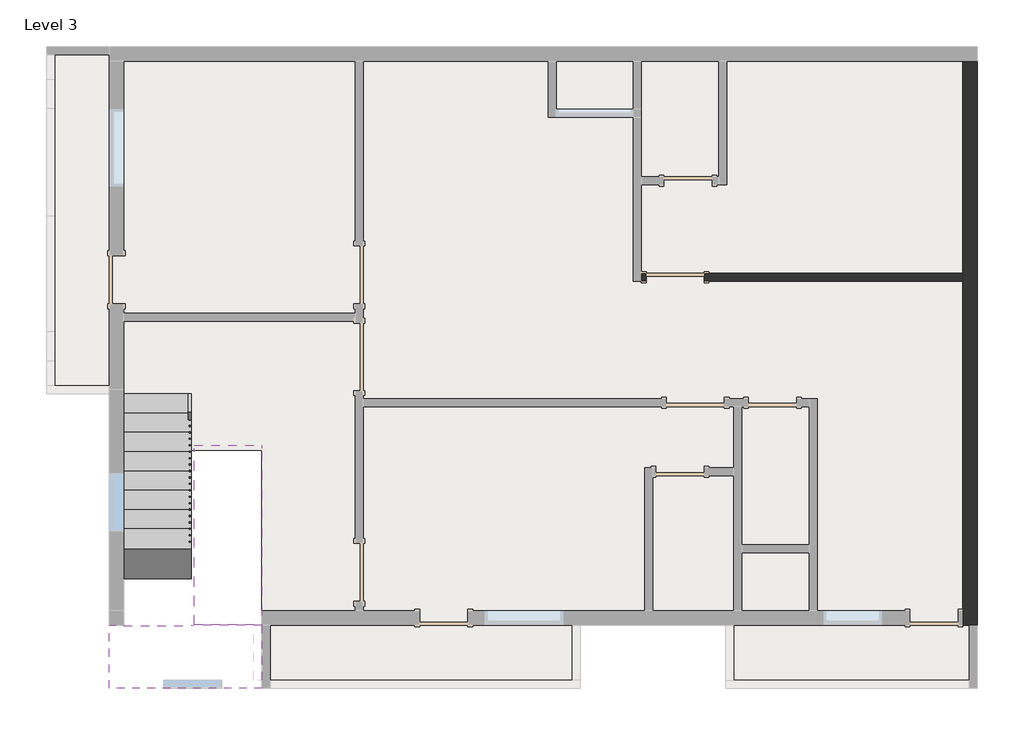
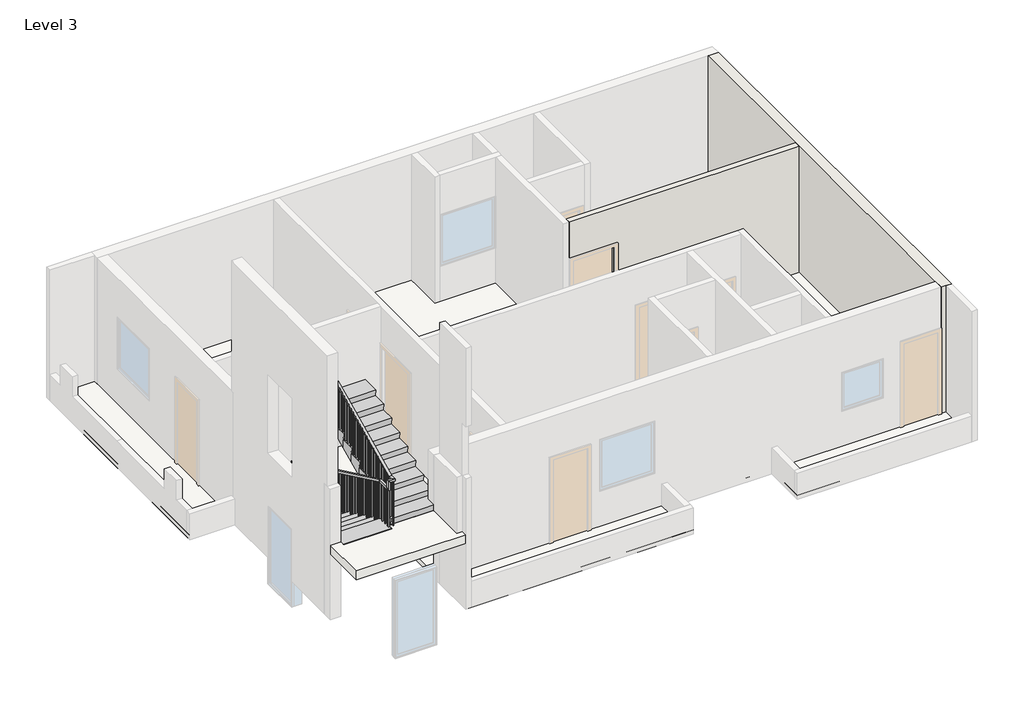
# One storey, part 2 of 2: 2 stair flights, 2 walls, 1 railing, 1 roof, 1 slab.
"""IFC4 building model written with IfcOpenShell, lengths in millimetres."""

from ifc_helpers import new_model, si_unit, frame, origin, place, context, project, spatial, polyline, outline, extrude, faceted_brep, element, save

model = new_model("IFC4")

# Units and contexts
model_context = context("Model", 3, world=origin())
ifc_project = project(units=[si_unit("LENGTHUNIT", "METRE", prefix="MILLI")], contexts=[model_context])

# Site, building, storey
site = spatial("IfcSite", under=ifc_project)
building = spatial("IfcBuilding", under=site)
storey = spatial("IfcBuildingStorey", under=building, Name="Level 3", Elevation=6096.0)

# Railing
placement = place(None, origin())
element("IfcRailing", 1, ObjectType="Handrail - Rectangular", at=placement, inside=storey, context=model_context, shape_type="SolidModel", body=[
    faceted_brep([(-9046.3394758, 7288.0495492, 7155.5428571), (-9046.3394758, 7288.0495492, 7099.2772447), (-9097.1394758, 7288.0495492, 7099.2772447), (-9097.1394758, 7288.0495492, 7155.5428571), (-9046.3394758, 3935.2495492, 8752.1142857), (-9046.3394758, 3923.7717632, 8701.3142857), (-9097.1394758, 3923.7717632, 8701.3142857), (-9097.1394758, 3935.2495492, 8752.1142857), (-9046.3394758, 3630.4495492, 8752.1142857), (-9097.1394758, 3630.4495492, 8752.1142857), (-9097.1394758, 3579.6495492, 8701.3142857), (-9046.3394758, 3579.6495492, 8701.3142857)], [[[0, 1, 2, 3]], [[1, 0, 4, 5]], [[2, 1, 5, 6]], [[3, 2, 6, 7]], [[0, 3, 7, 4]], [[8, 9, 10, 11]], [[5, 4, 8, 11]], [[6, 5, 11, 10]], [[7, 6, 10, 9]], [[4, 7, 9, 8]]]),
    faceted_brep([(-9046.3394758, 3630.4495492, 8752.1142857), (-9046.3394758, 3579.6495492, 8701.3142857), (-9097.1394758, 3579.6495492, 8701.3142857), (-9097.1394758, 3630.4495492, 8752.1142857), (-9046.3394758, 3630.4495492, 8882.7428571), (-9097.1394758, 3630.4495492, 8933.5428571), (-9097.1394758, 3579.6495492, 8933.5428571), (-9046.3394758, 3579.6495492, 8882.7428571)], [[[0, 1, 2, 3]], [[4, 5, 6, 7]], [[1, 0, 4, 7]], [[2, 1, 7, 6]], [[3, 2, 6, 5]], [[0, 3, 5, 4]]]),
    faceted_brep([(-9097.1394758, 3630.4495492, 8933.5428571), (-9046.3394758, 3630.4495492, 8882.7428571), (-9046.3394758, 3579.6495492, 8882.7428571), (-9097.1394758, 3579.6495492, 8933.5428571), (-8995.5394758, 3630.4495492, 8933.5428571), (-8995.5394758, 3630.4495492, 8882.7428571), (-8944.7394758, 3579.6495492, 8882.7428571), (-8944.7394758, 3579.6495492, 8933.5428571), (-8995.5394758, 3706.6495492, 8933.5428571), (-8995.5394758, 3718.1273353, 8882.7428571), (-8944.7394758, 3718.1273353, 8882.7428571), (-8944.7394758, 3706.6495492, 8933.5428571), (-8995.5394758, 6068.8495492, 10058.4), (-8995.5394758, 6080.3273353, 10007.6), (-8944.7394758, 6080.3273353, 10007.6), (-8944.7394758, 6068.8495492, 10058.4), (-8995.5394758, 6373.6495492, 10058.4), (-8944.7394758, 6373.6495492, 10058.4), (-8944.7394758, 6373.6495492, 10007.6), (-8995.5394758, 6373.6495492, 10007.6)], [[[0, 1, 2, 3]], [[1, 0, 4, 5]], [[2, 1, 5, 6]], [[3, 2, 6, 7]], [[0, 3, 7, 4]], [[5, 4, 8, 9]], [[6, 5, 9, 10]], [[7, 6, 10, 11]], [[4, 7, 11, 8]], [[9, 8, 12, 13]], [[10, 9, 13, 14]], [[11, 10, 14, 15]], [[8, 11, 15, 12]], [[16, 17, 18, 19]], [[13, 12, 16, 19]], [[14, 13, 19, 18]], [[15, 14, 18, 17]], [[12, 15, 17, 16]]]),
    extrude(outline(polyline([(-8979.6644758, 6338.7245492), (-8979.6644758, 6357.7745492), (-8960.6144758, 6357.7745492), (-8960.6144758, 6338.7245492), (-8979.6644758, 6338.7245492)])), frame((0.0, 0.0, 9144.0), z_axis=(0.0, 0.0, 1.0), x_axis=(1.0, 0.0, 0.0)), (0.0, 0.0, 1.0), 863.6),
    extrude(outline(polyline([(-8979.6644758, 6237.1245492), (-8979.6644758, 6256.1745492), (-8960.6144758, 6256.1745492), (-8960.6144758, 6237.1245492), (-8979.6644758, 6237.1245492)])), frame((0.0, 0.0, 9144.0), z_axis=(0.0, 0.0, 1.0), x_axis=(1.0, 0.0, 0.0)), (0.0, 0.0, 1.0), 863.6),
    extrude(outline(polyline([(-8979.6644758, 6135.5245492), (-8979.6644758, 6154.5745492), (-8960.6144758, 6154.5745492), (-8960.6144758, 6135.5245492), (-8979.6644758, 6135.5245492)])), frame((0.0, 0.0, 9144.0), z_axis=(0.0, 0.0, 1.0), x_axis=(1.0, 0.0, 0.0)), (0.0, 0.0, 1.0), 863.6),
    extrude(outline(polyline([(6052.9745492, 9994.5748638), (6052.9745492, 8998.8571429), (6033.9245492, 8998.8571429), (6033.9245492, 9985.5034352), (6052.9745492, 9994.5748638)])), frame((-8979.6644758, 0.0, 0.0), z_axis=(1.0, 0.0, 0.0), x_axis=(0.0, 1.0, 0.0)), (0.0, 0.0, 1.0), 19.05),
    extrude(outline(polyline([(5951.3745492, 9946.1939114), (5951.3745492, 8998.8571429), (5932.3245492, 8998.8571429), (5932.3245492, 9937.1224828), (5951.3745492, 9946.1939114)])), frame((-8979.6644758, 0.0, 0.0), z_axis=(1.0, 0.0, 0.0), x_axis=(0.0, 1.0, 0.0)), (0.0, 0.0, 1.0), 19.05),
    extrude(outline(polyline([(5849.7745492, 9897.812959), (5849.7745492, 8998.8571429), (5830.7245492, 8998.8571429), (5830.7245492, 9888.7415305), (5849.7745492, 9897.812959)])), frame((-8979.6644758, 0.0, 0.0), z_axis=(1.0, 0.0, 0.0), x_axis=(0.0, 1.0, 0.0)), (0.0, 0.0, 1.0), 19.05),
    extrude(outline(polyline([(5748.1745492, 9849.4320067), (5748.1745492, 8853.7142857), (5729.1245492, 8853.7142857), (5729.1245492, 9840.3605781), (5748.1745492, 9849.4320067)])), frame((-8979.6644758, 0.0, 0.0), z_axis=(1.0, 0.0, 0.0), x_axis=(0.0, 1.0, 0.0)), (0.0, 0.0, 1.0), 19.05),
    extrude(outline(polyline([(5646.5745492, 9801.0510543), (5646.5745492, 8853.7142857), (5627.5245492, 8853.7142857), (5627.5245492, 9791.9796257), (5646.5745492, 9801.0510543)])), frame((-8979.6644758, 0.0, 0.0), z_axis=(1.0, 0.0, 0.0), x_axis=(0.0, 1.0, 0.0)), (0.0, 0.0, 1.0), 19.05),
    extrude(outline(polyline([(5544.9745492, 9752.6701019), (5544.9745492, 8853.7142857), (5525.9245492, 8853.7142857), (5525.9245492, 9743.5986733), (5544.9745492, 9752.6701019)])), frame((-8979.6644758, 0.0, 0.0), z_axis=(1.0, 0.0, 0.0), x_axis=(0.0, 1.0, 0.0)), (0.0, 0.0, 1.0), 19.05),
    extrude(outline(polyline([(5443.3745492, 9704.2891495), (5443.3745492, 8708.5714286), (5424.3245492, 8708.5714286), (5424.3245492, 9695.2177209), (5443.3745492, 9704.2891495)])), frame((-8979.6644758, 0.0, 0.0), z_axis=(1.0, 0.0, 0.0), x_axis=(0.0, 1.0, 0.0)), (0.0, 0.0, 1.0), 19.05),
    extrude(outline(polyline([(5341.7745492, 9655.9081971), (5341.7745492, 8708.5714286), (5322.7245492, 8708.5714286), (5322.7245492, 9646.8367686), (5341.7745492, 9655.9081971)])), frame((-8979.6644758, 0.0, 0.0), z_axis=(1.0, 0.0, 0.0), x_axis=(0.0, 1.0, 0.0)), (0.0, 0.0, 1.0), 19.05),
    extrude(outline(polyline([(5240.1745492, 9607.5272447), (5240.1745492, 8708.5714286), (5221.1245492, 8708.5714286), (5221.1245492, 9598.4558162), (5240.1745492, 9607.5272447)])), frame((-8979.6644758, 0.0, 0.0), z_axis=(1.0, 0.0, 0.0), x_axis=(0.0, 1.0, 0.0)), (0.0, 0.0, 1.0), 19.05),
    extrude(outline(polyline([(5138.5745492, 9559.1462924), (5138.5745492, 8563.4285714), (5119.5245492, 8563.4285714), (5119.5245492, 9550.0748638), (5138.5745492, 9559.1462924)])), frame((-8979.6644758, 0.0, 0.0), z_axis=(1.0, 0.0, 0.0), x_axis=(0.0, 1.0, 0.0)), (0.0, 0.0, 1.0), 19.05),
    extrude(outline(polyline([(5036.9745492, 9510.76534), (5036.9745492, 8563.4285714), (5017.9245492, 8563.4285714), (5017.9245492, 9501.6939114), (5036.9745492, 9510.76534)])), frame((-8979.6644758, 0.0, 0.0), z_axis=(1.0, 0.0, 0.0), x_axis=(0.0, 1.0, 0.0)), (0.0, 0.0, 1.0), 19.05),
    extrude(outline(polyline([(4935.3745492, 9462.3843876), (4935.3745492, 8563.4285714), (4916.3245492, 8563.4285714), (4916.3245492, 9453.312959), (4935.3745492, 9462.3843876)])), frame((-8979.6644758, 0.0, 0.0), z_axis=(1.0, 0.0, 0.0), x_axis=(0.0, 1.0, 0.0)), (0.0, 0.0, 1.0), 19.05),
    extrude(outline(polyline([(4833.7745492, 9414.0034352), (4833.7745492, 8418.2857143), (4814.7245492, 8418.2857143), (4814.7245492, 9404.9320067), (4833.7745492, 9414.0034352)])), frame((-8979.6644758, 0.0, 0.0), z_axis=(1.0, 0.0, 0.0), x_axis=(0.0, 1.0, 0.0)), (0.0, 0.0, 1.0), 19.05),
    extrude(outline(polyline([(4732.1745492, 9365.6224828), (4732.1745492, 8418.2857143), (4713.1245492, 8418.2857143), (4713.1245492, 9356.5510543), (4732.1745492, 9365.6224828)])), frame((-8979.6644758, 0.0, 0.0), z_axis=(1.0, 0.0, 0.0), x_axis=(0.0, 1.0, 0.0)), (0.0, 0.0, 1.0), 19.05),
    extrude(outline(polyline([(4630.5745492, 9317.2415305), (4630.5745492, 8418.2857143), (4611.5245492, 8418.2857143), (4611.5245492, 9308.1701019), (4630.5745492, 9317.2415305)])), frame((-8979.6644758, 0.0, 0.0), z_axis=(1.0, 0.0, 0.0), x_axis=(0.0, 1.0, 0.0)), (0.0, 0.0, 1.0), 19.05),
    extrude(outline(polyline([(4528.9745492, 9268.8605781), (4528.9745492, 8273.1428571), (4509.9245492, 8273.1428571), (4509.9245492, 9259.7891495), (4528.9745492, 9268.8605781)])), frame((-8979.6644758, 0.0, 0.0), z_axis=(1.0, 0.0, 0.0), x_axis=(0.0, 1.0, 0.0)), (0.0, 0.0, 1.0), 19.05),
    extrude(outline(polyline([(4427.3745492, 9220.4796257), (4427.3745492, 8273.1428571), (4408.3245492, 8273.1428571), (4408.3245492, 9211.4081971), (4427.3745492, 9220.4796257)])), frame((-8979.6644758, 0.0, 0.0), z_axis=(1.0, 0.0, 0.0), x_axis=(0.0, 1.0, 0.0)), (0.0, 0.0, 1.0), 19.05),
    extrude(outline(polyline([(4325.7745492, 9172.0986733), (4325.7745492, 8273.1428571), (4306.7245492, 8273.1428571), (4306.7245492, 9163.0272447), (4325.7745492, 9172.0986733)])), frame((-8979.6644758, 0.0, 0.0), z_axis=(1.0, 0.0, 0.0), x_axis=(0.0, 1.0, 0.0)), (0.0, 0.0, 1.0), 19.05),
    extrude(outline(polyline([(4224.1745492, 9123.7177209), (4224.1745492, 8128.0), (4205.1245492, 8128.0), (4205.1245492, 9114.6462924), (4224.1745492, 9123.7177209)])), frame((-8979.6644758, 0.0, 0.0), z_axis=(1.0, 0.0, 0.0), x_axis=(0.0, 1.0, 0.0)), (0.0, 0.0, 1.0), 19.05),
    extrude(outline(polyline([(4122.5745492, 9075.3367686), (4122.5745492, 8128.0), (4103.5245492, 8128.0), (4103.5245492, 9066.26534), (4122.5745492, 9075.3367686)])), frame((-8979.6644758, 0.0, 0.0), z_axis=(1.0, 0.0, 0.0), x_axis=(0.0, 1.0, 0.0)), (0.0, 0.0, 1.0), 19.05),
    extrude(outline(polyline([(4020.9745492, 9026.9558162), (4020.9745492, 8128.0), (4001.9245492, 8128.0), (4001.9245492, 9017.8843876), (4020.9745492, 9026.9558162)])), frame((-8979.6644758, 0.0, 0.0), z_axis=(1.0, 0.0, 0.0), x_axis=(0.0, 1.0, 0.0)), (0.0, 0.0, 1.0), 19.05),
    extrude(outline(polyline([(3919.3745492, 8978.5748638), (3919.3745492, 7982.8571429), (3900.3245492, 7982.8571429), (3900.3245492, 8969.5034352), (3919.3745492, 8978.5748638)])), frame((-8979.6644758, 0.0, 0.0), z_axis=(1.0, 0.0, 0.0), x_axis=(0.0, 1.0, 0.0)), (0.0, 0.0, 1.0), 19.05),
    extrude(outline(polyline([(3817.7745492, 8930.1939114), (3817.7745492, 7982.8571429), (3798.7245492, 7982.8571429), (3798.7245492, 8921.1224828), (3817.7745492, 8930.1939114)])), frame((-8979.6644758, 0.0, 0.0), z_axis=(1.0, 0.0, 0.0), x_axis=(0.0, 1.0, 0.0)), (0.0, 0.0, 1.0), 19.05),
    extrude(outline(polyline([(3716.1745492, 8881.812959), (3716.1745492, 7982.8571429), (3697.1245492, 7982.8571429), (3697.1245492, 8872.7415305), (3716.1745492, 8881.812959)])), frame((-8979.6644758, 0.0, 0.0), z_axis=(1.0, 0.0, 0.0), x_axis=(0.0, 1.0, 0.0)), (0.0, 0.0, 1.0), 19.05),
    extrude(outline(polyline([(-9062.2144758, 3639.9745492), (-9062.2144758, 3620.9245492), (-9081.2644758, 3620.9245492), (-9081.2644758, 3639.9745492), (-9062.2144758, 3639.9745492)])), frame((0.0, 0.0, 7837.7142857), z_axis=(0.0, 0.0, 1.0), x_axis=(1.0, 0.0, 0.0)), (0.0, 0.0, 1.0), 863.6),
    extrude(outline(polyline([(-9062.2144758, 3741.5745492), (-9062.2144758, 3722.5245492), (-9081.2644758, 3722.5245492), (-9081.2644758, 3741.5745492), (-9062.2144758, 3741.5745492)])), frame((0.0, 0.0, 7837.7142857), z_axis=(0.0, 0.0, 1.0), x_axis=(1.0, 0.0, 0.0)), (0.0, 0.0, 1.0), 863.6),
    extrude(outline(polyline([(-9062.2144758, 3843.1745492), (-9062.2144758, 3824.1245492), (-9081.2644758, 3824.1245492), (-9081.2644758, 3843.1745492), (-9062.2144758, 3843.1745492)])), frame((0.0, 0.0, 7837.7142857), z_axis=(0.0, 0.0, 1.0), x_axis=(1.0, 0.0, 0.0)), (0.0, 0.0, 1.0), 863.6),
    extrude(outline(polyline([(3944.7745492, 8691.312959), (3944.7745492, 7837.7142857), (3925.7245492, 7837.7142857), (3925.7245492, 8700.3843876), (3944.7745492, 8691.312959)])), frame((-9081.2644758, 0.0, 0.0), z_axis=(1.0, 0.0, 0.0), x_axis=(0.0, 1.0, 0.0)), (0.0, 0.0, 1.0), 19.05),
    extrude(outline(polyline([(4046.3745492, 8642.9320067), (4046.3745492, 7692.5714286), (4027.3245492, 7692.5714286), (4027.3245492, 8652.0034352), (4046.3745492, 8642.9320067)])), frame((-9081.2644758, 0.0, 0.0), z_axis=(1.0, 0.0, 0.0), x_axis=(0.0, 1.0, 0.0)), (0.0, 0.0, 1.0), 19.05),
    extrude(outline(polyline([(4147.9745492, 8594.5510543), (4147.9745492, 7692.5714286), (4128.9245492, 7692.5714286), (4128.9245492, 8603.6224828), (4147.9745492, 8594.5510543)])), frame((-9081.2644758, 0.0, 0.0), z_axis=(1.0, 0.0, 0.0), x_axis=(0.0, 1.0, 0.0)), (0.0, 0.0, 1.0), 19.05),
    extrude(outline(polyline([(4249.5745492, 8546.1701019), (4249.5745492, 7692.5714286), (4230.5245492, 7692.5714286), (4230.5245492, 8555.2415305), (4249.5745492, 8546.1701019)])), frame((-9081.2644758, 0.0, 0.0), z_axis=(1.0, 0.0, 0.0), x_axis=(0.0, 1.0, 0.0)), (0.0, 0.0, 1.0), 19.05),
    extrude(outline(polyline([(4351.1745492, 8497.7891495), (4351.1745492, 7547.4285714), (4332.1245492, 7547.4285714), (4332.1245492, 8506.8605781), (4351.1745492, 8497.7891495)])), frame((-9081.2644758, 0.0, 0.0), z_axis=(1.0, 0.0, 0.0), x_axis=(0.0, 1.0, 0.0)), (0.0, 0.0, 1.0), 19.05),
    extrude(outline(polyline([(4452.7745492, 8449.4081971), (4452.7745492, 7547.4285714), (4433.7245492, 7547.4285714), (4433.7245492, 8458.4796257), (4452.7745492, 8449.4081971)])), frame((-9081.2644758, 0.0, 0.0), z_axis=(1.0, 0.0, 0.0), x_axis=(0.0, 1.0, 0.0)), (0.0, 0.0, 1.0), 19.05),
    extrude(outline(polyline([(4554.3745492, 8401.0272447), (4554.3745492, 7547.4285714), (4535.3245492, 7547.4285714), (4535.3245492, 8410.0986733), (4554.3745492, 8401.0272447)])), frame((-9081.2644758, 0.0, 0.0), z_axis=(1.0, 0.0, 0.0), x_axis=(0.0, 1.0, 0.0)), (0.0, 0.0, 1.0), 19.05),
    extrude(outline(polyline([(4655.9745492, 8352.6462924), (4655.9745492, 7402.2857143), (4636.9245492, 7402.2857143), (4636.9245492, 8361.7177209), (4655.9745492, 8352.6462924)])), frame((-9081.2644758, 0.0, 0.0), z_axis=(1.0, 0.0, 0.0), x_axis=(0.0, 1.0, 0.0)), (0.0, 0.0, 1.0), 19.05),
    extrude(outline(polyline([(4757.5745492, 8304.26534), (4757.5745492, 7402.2857143), (4738.5245492, 7402.2857143), (4738.5245492, 8313.3367686), (4757.5745492, 8304.26534)])), frame((-9081.2644758, 0.0, 0.0), z_axis=(1.0, 0.0, 0.0), x_axis=(0.0, 1.0, 0.0)), (0.0, 0.0, 1.0), 19.05),
    extrude(outline(polyline([(4859.1745492, 8255.8843876), (4859.1745492, 7402.2857143), (4840.1245492, 7402.2857143), (4840.1245492, 8264.9558162), (4859.1745492, 8255.8843876)])), frame((-9081.2644758, 0.0, 0.0), z_axis=(1.0, 0.0, 0.0), x_axis=(0.0, 1.0, 0.0)), (0.0, 0.0, 1.0), 19.05),
    extrude(outline(polyline([(4960.7745492, 8207.5034352), (4960.7745492, 7257.1428571), (4941.7245492, 7257.1428571), (4941.7245492, 8216.5748638), (4960.7745492, 8207.5034352)])), frame((-9081.2644758, 0.0, 0.0), z_axis=(1.0, 0.0, 0.0), x_axis=(0.0, 1.0, 0.0)), (0.0, 0.0, 1.0), 19.05),
    extrude(outline(polyline([(5062.3745492, 8159.1224828), (5062.3745492, 7257.1428571), (5043.3245492, 7257.1428571), (5043.3245492, 8168.1939114), (5062.3745492, 8159.1224828)])), frame((-9081.2644758, 0.0, 0.0), z_axis=(1.0, 0.0, 0.0), x_axis=(0.0, 1.0, 0.0)), (0.0, 0.0, 1.0), 19.05),
    extrude(outline(polyline([(5163.9745492, 8110.7415305), (5163.9745492, 7257.1428571), (5144.9245492, 7257.1428571), (5144.9245492, 8119.812959), (5163.9745492, 8110.7415305)])), frame((-9081.2644758, 0.0, 0.0), z_axis=(1.0, 0.0, 0.0), x_axis=(0.0, 1.0, 0.0)), (0.0, 0.0, 1.0), 19.05),
    extrude(outline(polyline([(5265.5745492, 8062.3605781), (5265.5745492, 7112.0), (5246.5245492, 7112.0), (5246.5245492, 8071.4320067), (5265.5745492, 8062.3605781)])), frame((-9081.2644758, 0.0, 0.0), z_axis=(1.0, 0.0, 0.0), x_axis=(0.0, 1.0, 0.0)), (0.0, 0.0, 1.0), 19.05),
    extrude(outline(polyline([(5367.1745492, 8013.9796257), (5367.1745492, 7112.0), (5348.1245492, 7112.0), (5348.1245492, 8023.0510543), (5367.1745492, 8013.9796257)])), frame((-9081.2644758, 0.0, 0.0), z_axis=(1.0, 0.0, 0.0), x_axis=(0.0, 1.0, 0.0)), (0.0, 0.0, 1.0), 19.05),
    extrude(outline(polyline([(5468.7745492, 7965.5986733), (5468.7745492, 7112.0), (5449.7245492, 7112.0), (5449.7245492, 7974.6701019), (5468.7745492, 7965.5986733)])), frame((-9081.2644758, 0.0, 0.0), z_axis=(1.0, 0.0, 0.0), x_axis=(0.0, 1.0, 0.0)), (0.0, 0.0, 1.0), 19.05),
    extrude(outline(polyline([(5570.3745492, 7917.2177209), (5570.3745492, 6966.8571429), (5551.3245492, 6966.8571429), (5551.3245492, 7926.2891495), (5570.3745492, 7917.2177209)])), frame((-9081.2644758, 0.0, 0.0), z_axis=(1.0, 0.0, 0.0), x_axis=(0.0, 1.0, 0.0)), (0.0, 0.0, 1.0), 19.05),
    extrude(outline(polyline([(5671.9745492, 7868.8367686), (5671.9745492, 6966.8571429), (5652.9245492, 6966.8571429), (5652.9245492, 7877.9081971), (5671.9745492, 7868.8367686)])), frame((-9081.2644758, 0.0, 0.0), z_axis=(1.0, 0.0, 0.0), x_axis=(0.0, 1.0, 0.0)), (0.0, 0.0, 1.0), 19.05),
    extrude(outline(polyline([(5773.5745492, 7820.4558162), (5773.5745492, 6966.8571429), (5754.5245492, 6966.8571429), (5754.5245492, 7829.5272447), (5773.5745492, 7820.4558162)])), frame((-9081.2644758, 0.0, 0.0), z_axis=(1.0, 0.0, 0.0), x_axis=(0.0, 1.0, 0.0)), (0.0, 0.0, 1.0), 19.05),
    extrude(outline(polyline([(5875.1745492, 7772.0748638), (5875.1745492, 6821.7142857), (5856.1245492, 6821.7142857), (5856.1245492, 7781.1462924), (5875.1745492, 7772.0748638)])), frame((-9081.2644758, 0.0, 0.0), z_axis=(1.0, 0.0, 0.0), x_axis=(0.0, 1.0, 0.0)), (0.0, 0.0, 1.0), 19.05),
    extrude(outline(polyline([(5976.7745492, 7723.6939114), (5976.7745492, 6821.7142857), (5957.7245492, 6821.7142857), (5957.7245492, 7732.76534), (5976.7745492, 7723.6939114)])), frame((-9081.2644758, 0.0, 0.0), z_axis=(1.0, 0.0, 0.0), x_axis=(0.0, 1.0, 0.0)), (0.0, 0.0, 1.0), 19.05),
    extrude(outline(polyline([(6078.3745492, 7675.312959), (6078.3745492, 6821.7142857), (6059.3245492, 6821.7142857), (6059.3245492, 7684.3843876), (6078.3745492, 7675.312959)])), frame((-9081.2644758, 0.0, 0.0), z_axis=(1.0, 0.0, 0.0), x_axis=(0.0, 1.0, 0.0)), (0.0, 0.0, 1.0), 19.05),
    extrude(outline(polyline([(6179.9745492, 7626.9320067), (6179.9745492, 6676.5714286), (6160.9245492, 6676.5714286), (6160.9245492, 7636.0034352), (6179.9745492, 7626.9320067)])), frame((-9081.2644758, 0.0, 0.0), z_axis=(1.0, 0.0, 0.0), x_axis=(0.0, 1.0, 0.0)), (0.0, 0.0, 1.0), 19.05),
    extrude(outline(polyline([(6281.5745492, 7578.5510543), (6281.5745492, 6676.5714286), (6262.5245492, 6676.5714286), (6262.5245492, 7587.6224828), (6281.5745492, 7578.5510543)])), frame((-9081.2644758, 0.0, 0.0), z_axis=(1.0, 0.0, 0.0), x_axis=(0.0, 1.0, 0.0)), (0.0, 0.0, 1.0), 19.05),
    extrude(outline(polyline([(6383.1745492, 7530.1701019), (6383.1745492, 6676.5714286), (6364.1245492, 6676.5714286), (6364.1245492, 7539.2415305), (6383.1745492, 7530.1701019)])), frame((-9081.2644758, 0.0, 0.0), z_axis=(1.0, 0.0, 0.0), x_axis=(0.0, 1.0, 0.0)), (0.0, 0.0, 1.0), 19.05),
    extrude(outline(polyline([(6484.7745492, 7481.7891495), (6484.7745492, 6531.4285714), (6465.7245492, 6531.4285714), (6465.7245492, 7490.8605781), (6484.7745492, 7481.7891495)])), frame((-9081.2644758, 0.0, 0.0), z_axis=(1.0, 0.0, 0.0), x_axis=(0.0, 1.0, 0.0)), (0.0, 0.0, 1.0), 19.05),
    extrude(outline(polyline([(6586.3745492, 7433.4081971), (6586.3745492, 6531.4285714), (6567.3245492, 6531.4285714), (6567.3245492, 7442.4796257), (6586.3745492, 7433.4081971)])), frame((-9081.2644758, 0.0, 0.0), z_axis=(1.0, 0.0, 0.0), x_axis=(0.0, 1.0, 0.0)), (0.0, 0.0, 1.0), 19.05),
    extrude(outline(polyline([(6687.9745492, 7385.0272447), (6687.9745492, 6531.4285714), (6668.9245492, 6531.4285714), (6668.9245492, 7394.0986733), (6687.9745492, 7385.0272447)])), frame((-9081.2644758, 0.0, 0.0), z_axis=(1.0, 0.0, 0.0), x_axis=(0.0, 1.0, 0.0)), (0.0, 0.0, 1.0), 19.05),
    extrude(outline(polyline([(6789.5745492, 7336.6462924), (6789.5745492, 6386.2857143), (6770.5245492, 6386.2857143), (6770.5245492, 7345.7177209), (6789.5745492, 7336.6462924)])), frame((-9081.2644758, 0.0, 0.0), z_axis=(1.0, 0.0, 0.0), x_axis=(0.0, 1.0, 0.0)), (0.0, 0.0, 1.0), 19.05),
    extrude(outline(polyline([(6891.1745492, 7288.26534), (6891.1745492, 6386.2857143), (6872.1245492, 6386.2857143), (6872.1245492, 7297.3367686), (6891.1745492, 7288.26534)])), frame((-9081.2644758, 0.0, 0.0), z_axis=(1.0, 0.0, 0.0), x_axis=(0.0, 1.0, 0.0)), (0.0, 0.0, 1.0), 19.05),
    extrude(outline(polyline([(6992.7745492, 7239.8843876), (6992.7745492, 6386.2857143), (6973.7245492, 6386.2857143), (6973.7245492, 7248.9558162), (6992.7745492, 7239.8843876)])), frame((-9081.2644758, 0.0, 0.0), z_axis=(1.0, 0.0, 0.0), x_axis=(0.0, 1.0, 0.0)), (0.0, 0.0, 1.0), 19.05),
    extrude(outline(polyline([(7094.3745492, 7191.5034352), (7094.3745492, 6241.1428571), (7075.3245492, 6241.1428571), (7075.3245492, 7200.5748638), (7094.3745492, 7191.5034352)])), frame((-9081.2644758, 0.0, 0.0), z_axis=(1.0, 0.0, 0.0), x_axis=(0.0, 1.0, 0.0)), (0.0, 0.0, 1.0), 19.05),
    extrude(outline(polyline([(7195.9745492, 7143.1224828), (7195.9745492, 6241.1428571), (7176.9245492, 6241.1428571), (7176.9245492, 7152.1939114), (7195.9745492, 7143.1224828)])), frame((-9081.2644758, 0.0, 0.0), z_axis=(1.0, 0.0, 0.0), x_axis=(0.0, 1.0, 0.0)), (0.0, 0.0, 1.0), 19.05),
    extrude(outline(polyline([(-8979.6644758, 3614.5745492), (-8960.6144758, 3614.5745492), (-8960.6144758, 3595.5245492), (-8979.6644758, 3595.5245492), (-8979.6644758, 3614.5745492)])), frame((0.0, 0.0, 7837.7142857), z_axis=(0.0, 0.0, 1.0), x_axis=(1.0, 0.0, 0.0)), (0.0, 0.0, 1.0), 1045.0285714),
    extrude(outline(polyline([(-9062.2144758, 3614.5745492), (-9062.2144758, 3595.5245492), (-9081.2644758, 3595.5245492), (-9081.2644758, 3614.5745492), (-9062.2144758, 3614.5745492)])), frame((0.0, 0.0, 7837.7142857), z_axis=(0.0, 0.0, 1.0), x_axis=(1.0, 0.0, 0.0)), (0.0, 0.0, 1.0), 863.6),
    extrude(outline(polyline([(-8979.6644758, 6354.5995492), (-8979.6644758, 6373.6495492), (-8960.6144758, 6373.6495492), (-8960.6144758, 6354.5995492), (-8979.6644758, 6354.5995492)])), frame((0.0, 0.0, 9144.0), z_axis=(0.0, 0.0, 1.0), x_axis=(1.0, 0.0, 0.0)), (0.0, 0.0, 1.0), 863.6),
    extrude(outline(polyline([(7288.0495492, 7099.2772447), (7288.0495492, 6241.1428571), (7268.9995492, 6241.1428571), (7268.9995492, 7108.3486733), (7288.0495492, 7099.2772447)])), frame((-9081.2644758, 0.0, 0.0), z_axis=(1.0, 0.0, 0.0), x_axis=(0.0, 1.0, 0.0)), (0.0, 0.0, 1.0), 19.05),
])

# Roof
element("IfcRoof", 2, ObjectType="Generic - 4\"", at=placement, inside=storey, context=model_context, shape_type="SweptSolid", body=[
    extrude(outline(polyline([(3374.2605242, 2639.8495492), (-600.8394758, 2639.8495492), (-600.8394758, 3630.4495492), (-2899.5394758, 3630.4495492), (-2899.5394758, 2639.8495492), (-7928.7394758, 2639.8495492), (-7928.7394758, 6399.0495492), (-9046.3394758, 6399.0495492), (-9046.3394758, 7288.0495492), (-11332.3394758, 7288.0495492), (-11332.3394758, 12774.4495492), (3374.2605242, 12774.4495492), (3374.2605242, 2639.8495492)])), frame((0.0, 0.0, 6096.0), z_axis=(0.0, 0.0, 1.0), x_axis=(1.0, 0.0, 0.0)), (0.0, 0.0, 1.0), 101.6),
])

# Slab
element("IfcSlab", 3, ObjectType="8\" Thickness", at=placement, inside=storey, context=model_context, shape_type="Brep", body=[
    faceted_brep([(-10341.7394758, 3630.4495492, 7837.7142857), (-10341.7394758, 2639.8495492, 7837.7142857), (-7928.7394758, 2639.8495492, 7837.7142857), (-7928.7394758, 3630.4495492, 7837.7142857), (-7928.7394758, 3649.4995492, 7837.7142857), (-8995.5394758, 3649.4995492, 7837.7142857), (-8995.5394758, 3630.4495492, 7837.7142857), (-9044.7519758, 3630.4495492, 7837.7142857), (-9044.7519758, 3519.3245492, 7837.7142857), (-10114.7269758, 3519.3245492, 7837.7142857), (-10114.7269758, 3630.4495492, 7837.7142857), (-10341.7394758, 3630.4495492, 7634.5142857), (-10341.7394758, 2639.8495492, 7634.5142857), (-7928.7394758, 2639.8495492, 7634.5142857), (-10114.7269758, 3630.4495492, 7634.5142857), (-10114.7269758, 3620.9245492, 7634.5142857), (-9044.7519758, 3620.9245492, 7634.5142857), (-9044.7519758, 3630.4495492, 7634.5142857), (-8995.5394758, 3630.4495492, 7634.5142857), (-8995.5394758, 3649.4995492, 7634.5142857), (-7928.7394758, 3649.4995492, 7634.5142857), (-7928.7394758, 3630.4495492, 7634.5142857), (-10114.7269758, 3519.3245492, 7726.5892857), (-9044.7519758, 3519.3245492, 7726.5892857), (-9044.7519758, 3620.9245492, 7726.5892857), (-10114.7269758, 3620.9245492, 7726.5892857)], [[[0, 1, 2, 3, 4, 5, 6, 7, 8, 9, 10]], [[1, 0, 11, 12]], [[2, 1, 12, 13]], [[12, 11, 14, 15, 16, 17, 18, 19, 20, 21, 13]], [[3, 2, 13, 21]], [[5, 4, 20, 19]], [[6, 18, 17, 7]], [[22, 23, 24, 25]], [[9, 22, 25, 15, 14, 10]], [[23, 22, 9, 8]], [[23, 8, 7, 17, 16, 24]], [[25, 24, 16, 15]], [[11, 0, 10, 14]], [[4, 3, 21, 20]], [[6, 5, 19, 18]]]),
])

# Stair flights
element("IfcStairFlight", 4, ObjectType="3/4\" Nosing 6 1/2\" Depth", at=placement, inside=storey, context=model_context, shape_type="Brep", body=[
    faceted_brep([(-10113.1394758, 7288.0495492, 6241.1428571), (-9046.3394758, 7288.0495492, 6241.1428571), (-9046.3394758, 7268.9995492, 6096.0), (-10113.1394758, 7268.9995492, 6096.0), (-10113.1394758, 6964.1995492, 6241.1428571), (-9046.3394758, 6964.1995492, 6241.1428571), (-9046.3394758, 6964.1995492, 6096.0), (-10113.1394758, 6964.1995492, 6096.0), (-9046.3394758, 6983.2495492, 6386.2857143), (-10113.1394758, 6983.2495492, 6386.2857143), (-10113.1394758, 6659.3995492, 6386.2857143), (-9046.3394758, 6659.3995492, 6386.2857143), (-9046.3394758, 6659.3995492, 6203.422474), (-9046.3394758, 6884.9867446, 6096.0), (-10113.1394758, 6884.9867446, 6096.0), (-10113.1394758, 6659.3995492, 6203.422474), (-9046.3394758, 6678.4495492, 6531.4285714), (-10113.1394758, 6678.4495492, 6531.4285714), (-10113.1394758, 6354.5995492, 6531.4285714), (-9046.3394758, 6354.5995492, 6531.4285714), (-9046.3394758, 6354.5995492, 6348.5653311), (-10113.1394758, 6354.5995492, 6348.5653311), (-9046.3394758, 6373.6495492, 6676.5714286), (-10113.1394758, 6373.6495492, 6676.5714286), (-10113.1394758, 6049.7995492, 6676.5714286), (-9046.3394758, 6049.7995492, 6676.5714286), (-9046.3394758, 6049.7995492, 6493.7081883), (-10113.1394758, 6049.7995492, 6493.7081883), (-9046.3394758, 6068.8495492, 6821.7142857), (-10113.1394758, 6068.8495492, 6821.7142857), (-10113.1394758, 5744.9995492, 6821.7142857), (-9046.3394758, 5744.9995492, 6821.7142857), (-9046.3394758, 5744.9995492, 6638.8510454), (-10113.1394758, 5744.9995492, 6638.8510454), (-9046.3394758, 5764.0495492, 6966.8571429), (-10113.1394758, 5764.0495492, 6966.8571429), (-10113.1394758, 5440.1995492, 6966.8571429), (-9046.3394758, 5440.1995492, 6966.8571429), (-9046.3394758, 5440.1995492, 6783.9939026), (-10113.1394758, 5440.1995492, 6783.9939026), (-9046.3394758, 5459.2495492, 7112.0), (-10113.1394758, 5459.2495492, 7112.0), (-10113.1394758, 5135.3995492, 7112.0), (-9046.3394758, 5135.3995492, 7112.0), (-9046.3394758, 5135.3995492, 6929.1367597), (-10113.1394758, 5135.3995492, 6929.1367597), (-9046.3394758, 5154.4495492, 7257.1428571), (-10113.1394758, 5154.4495492, 7257.1428571), (-10113.1394758, 4830.5995492, 7257.1428571), (-9046.3394758, 4830.5995492, 7257.1428571), (-9046.3394758, 4830.5995492, 7074.2796169), (-10113.1394758, 4830.5995492, 7074.2796169), (-9046.3394758, 4849.6495492, 7402.2857143), (-10113.1394758, 4849.6495492, 7402.2857143), (-10113.1394758, 4525.7995492, 7402.2857143), (-9046.3394758, 4525.7995492, 7402.2857143), (-9046.3394758, 4525.7995492, 7219.422474), (-10113.1394758, 4525.7995492, 7219.422474), (-9046.3394758, 4544.8495492, 7547.4285714), (-10113.1394758, 4544.8495492, 7547.4285714), (-10113.1394758, 4220.9995492, 7547.4285714), (-9046.3394758, 4220.9995492, 7547.4285714), (-9046.3394758, 4220.9995492, 7364.5653311), (-10113.1394758, 4220.9995492, 7364.5653311), (-9046.3394758, 4240.0495492, 7692.5714286), (-10113.1394758, 4240.0495492, 7692.5714286), (-10113.1394758, 3916.1995492, 7692.5714286), (-9046.3394758, 3916.1995492, 7692.5714286), (-9046.3394758, 3916.1995492, 7509.7081883), (-10113.1394758, 3916.1995492, 7509.7081883), (-9046.3394758, 3935.2495492, 7837.7142857), (-10113.1394758, 3935.2495492, 7837.7142857), (-10113.1394758, 3528.8495492, 7837.7142857), (-9046.3394758, 3528.8495492, 7837.7142857), (-9046.3394758, 3528.8495492, 7736.1142857), (-9046.3394758, 3630.4495492, 7736.1142857), (-9046.3394758, 3630.4495492, 7634.5142857), (-9046.3394758, 3654.1067446, 7634.5142857), (-10113.1394758, 3654.1067446, 7634.5142857), (-10113.1394758, 3630.4495492, 7634.5142857), (-10113.1394758, 3630.4495492, 7736.1142857), (-10113.1394758, 3528.8495492, 7736.1142857)], [[[0, 1, 2, 3]], [[1, 0, 4, 5]], [[1, 5, 6, 2]], [[4, 0, 3, 7]], [[8, 9, 10, 11]], [[6, 5, 8, 11, 12, 13]], [[4, 7, 14, 15, 10, 9]], [[5, 4, 9, 8]], [[16, 17, 18, 19]], [[16, 19, 20, 12, 11]], [[18, 17, 10, 15, 21]], [[11, 10, 17, 16]], [[22, 23, 24, 25]], [[22, 25, 26, 20, 19]], [[24, 23, 18, 21, 27]], [[19, 18, 23, 22]], [[28, 29, 30, 31]], [[28, 31, 32, 26, 25]], [[30, 29, 24, 27, 33]], [[25, 24, 29, 28]], [[34, 35, 36, 37]], [[34, 37, 38, 32, 31]], [[36, 35, 30, 33, 39]], [[31, 30, 35, 34]], [[40, 41, 42, 43]], [[40, 43, 44, 38, 37]], [[42, 41, 36, 39, 45]], [[37, 36, 41, 40]], [[46, 47, 48, 49]], [[46, 49, 50, 44, 43]], [[48, 47, 42, 45, 51]], [[43, 42, 47, 46]], [[52, 53, 54, 55]], [[52, 55, 56, 50, 49]], [[54, 53, 48, 51, 57]], [[49, 48, 53, 52]], [[58, 59, 60, 61]], [[58, 61, 62, 56, 55]], [[60, 59, 54, 57, 63]], [[55, 54, 59, 58]], [[64, 65, 66, 67]], [[64, 67, 68, 62, 61]], [[66, 65, 60, 63, 69]], [[61, 60, 65, 64]], [[70, 71, 72, 73]], [[67, 70, 73, 74, 75, 76, 77, 68]], [[72, 71, 66, 69, 78, 79, 80, 81]], [[79, 76, 75, 80]], [[67, 66, 71, 70]], [[2, 6, 13, 14, 7, 3]], [[77, 78, 69, 63, 57, 51, 45, 39, 33, 27, 21, 15, 14, 13, 12, 20, 26, 32, 38, 44, 50, 56, 62, 68]], [[81, 80, 75, 74]], [[81, 74, 73, 72]], [[78, 77, 76, 79]]]),
])
element("IfcStairFlight", 5, ObjectType="3/4\" Nosing 6 1/2\" Depth", at=placement, inside=storey, context=model_context, shape_type="Brep", body=[
    faceted_brep([(-7928.7394758, 3630.4495492, 7982.8571429), (-8995.5394758, 3630.4495492, 7982.8571429), (-8995.5394758, 3649.4995492, 7837.7142857), (-7928.7394758, 3649.4995492, 7837.7142857), (-7928.7394758, 3954.2995492, 7982.8571429), (-8995.5394758, 3954.2995492, 7982.8571429), (-8995.5394758, 3954.2995492, 7799.9939026), (-8995.5394758, 3649.4995492, 7654.8510454), (-7928.7394758, 3649.4995492, 7654.8510454), (-7928.7394758, 3954.2995492, 7799.9939026), (-8995.5394758, 3935.2495492, 8128.0), (-7928.7394758, 3935.2495492, 8128.0), (-7928.7394758, 4259.0995492, 8128.0), (-8995.5394758, 4259.0995492, 8128.0), (-8995.5394758, 4259.0995492, 7945.1367597), (-7928.7394758, 4259.0995492, 7945.1367597), (-8995.5394758, 4240.0495492, 8273.1428571), (-7928.7394758, 4240.0495492, 8273.1428571), (-7928.7394758, 4563.8995492, 8273.1428571), (-8995.5394758, 4563.8995492, 8273.1428571), (-8995.5394758, 4563.8995492, 8090.2796169), (-7928.7394758, 4563.8995492, 8090.2796169), (-8995.5394758, 4544.8495492, 8418.2857143), (-7928.7394758, 4544.8495492, 8418.2857143), (-7928.7394758, 4868.6995492, 8418.2857143), (-8995.5394758, 4868.6995492, 8418.2857143), (-8995.5394758, 4868.6995492, 8235.422474), (-7928.7394758, 4868.6995492, 8235.422474), (-8995.5394758, 4849.6495492, 8563.4285714), (-7928.7394758, 4849.6495492, 8563.4285714), (-7928.7394758, 5173.4995492, 8563.4285714), (-8995.5394758, 5173.4995492, 8563.4285714), (-8995.5394758, 5173.4995492, 8380.5653311), (-7928.7394758, 5173.4995492, 8380.5653311), (-8995.5394758, 5154.4495492, 8708.5714286), (-7928.7394758, 5154.4495492, 8708.5714286), (-7928.7394758, 5478.2995492, 8708.5714286), (-8995.5394758, 5478.2995492, 8708.5714286), (-8995.5394758, 5478.2995492, 8525.7081883), (-7928.7394758, 5478.2995492, 8525.7081883), (-8995.5394758, 5459.2495492, 8853.7142857), (-7928.7394758, 5459.2495492, 8853.7142857), (-7928.7394758, 5783.0995492, 8853.7142857), (-8995.5394758, 5783.0995492, 8853.7142857), (-8995.5394758, 5783.0995492, 8670.8510454), (-7928.7394758, 5783.0995492, 8670.8510454), (-8995.5394758, 5764.0495492, 8998.8571429), (-7928.7394758, 5764.0495492, 8998.8571429), (-7928.7394758, 6087.8995492, 8998.8571429), (-8995.5394758, 6087.8995492, 8998.8571429), (-8995.5394758, 6087.8995492, 8815.9939026), (-7928.7394758, 6087.8995492, 8815.9939026), (-8995.5394758, 6068.8495492, 9144.0), (-7928.7394758, 6068.8495492, 9144.0), (-7928.7394758, 6475.2495492, 9144.0), (-8995.5394758, 6475.2495492, 9144.0), (-8995.5394758, 6475.2495492, 9042.4), (-8995.5394758, 6373.6495492, 9042.4), (-8995.5394758, 6373.6495492, 8952.0653311), (-7928.7394758, 6373.6495492, 8952.0653311), (-7928.7394758, 6373.6495492, 9042.4), (-7928.7394758, 6475.2495492, 9042.4)], [[[0, 1, 2, 3]], [[1, 0, 4, 5]], [[1, 5, 6, 7, 2]], [[3, 2, 7, 8]], [[4, 0, 3, 8, 9]], [[10, 11, 12, 13]], [[10, 13, 14, 6, 5]], [[12, 11, 4, 9, 15]], [[11, 10, 5, 4]], [[16, 17, 18, 19]], [[16, 19, 20, 14, 13]], [[18, 17, 12, 15, 21]], [[17, 16, 13, 12]], [[22, 23, 24, 25]], [[22, 25, 26, 20, 19]], [[24, 23, 18, 21, 27]], [[23, 22, 19, 18]], [[28, 29, 30, 31]], [[28, 31, 32, 26, 25]], [[30, 29, 24, 27, 33]], [[29, 28, 25, 24]], [[34, 35, 36, 37]], [[34, 37, 38, 32, 31]], [[36, 35, 30, 33, 39]], [[35, 34, 31, 30]], [[40, 41, 42, 43]], [[40, 43, 44, 38, 37]], [[42, 41, 36, 39, 45]], [[41, 40, 37, 36]], [[46, 47, 48, 49]], [[46, 49, 50, 44, 43]], [[48, 47, 42, 45, 51]], [[47, 46, 43, 42]], [[52, 53, 54, 55]], [[52, 55, 56, 57, 58, 50, 49]], [[54, 53, 48, 51, 59, 60, 61]], [[59, 58, 57, 60]], [[53, 52, 49, 48]], [[7, 6, 14, 20, 26, 32, 38, 44, 50, 58, 59, 51, 45, 39, 33, 27, 21, 15, 9, 8]], [[61, 60, 57, 56]], [[61, 56, 55, 54]]]),
])

# Walls
element("IfcWall", 6, ObjectType="Generic - 5\"", at=placement, inside=storey, context=model_context, shape_type="SweptSolid", body=[
    extrude(outline(polyline([(6096.0, -1934.3394758), (6096.0, -1858.1394758), (8229.6, -1858.1394758), (8229.6, -943.7394758), (6096.0, -943.7394758), (6096.0, 3145.6605242), (9144.0, 3145.6605242), (9144.0, -1934.3394758), (6096.0, -1934.3394758)])), frame((0.0, 9066.0495492, 0.0), z_axis=(0.0, 1.0, 0.0), x_axis=(0.0, 0.0, 1.0)), (0.0, 0.0, 1.0), 127.0),
])
element("IfcWall", 7, ObjectType="Generic - 9\"", at=placement, inside=storey, context=model_context, shape_type="Brep", body=[
    faceted_brep([(3145.6605242, 12545.8495492, 6096.0), (3145.6605242, 9193.0495492, 6096.0), (3145.6605242, 9066.0495492, 6096.0), (3145.6605242, 3859.0495492, 6096.0), (3145.6605242, 3630.4495492, 6096.0), (3145.6605242, 3630.4495492, 9144.0), (3145.6605242, 3859.0495492, 9144.0), (3145.6605242, 9066.0495492, 9144.0), (3145.6605242, 9193.0495492, 9144.0), (3145.6605242, 12545.8495492, 9144.0), (3374.2605242, 12545.8495492, 6096.0), (3374.2605242, 12545.8495492, 9144.0), (3374.2605242, 3630.4495492, 9144.0), (3374.2605242, 3630.4495492, 6096.0), (3247.2605242, 3630.4495492, 6096.0), (3247.2605242, 3630.4495492, 9144.0)], [[[0, 1, 2, 3, 4, 5, 6, 7, 8, 9]], [[10, 11, 12, 13]], [[4, 3, 2, 1, 0, 10, 13, 14]], [[9, 8, 7, 6, 5, 15, 12, 11]], [[0, 9, 11, 10]], [[5, 4, 14, 13, 12, 15]]]),
])

save(model, "model.ifc")

# Revit data of these elements
# Type "Handrail - Rectangular"
#   Assembly Code = "C2010400"
#   built-in parameter 1008612 = 0.0416667 (stored number, unit not read)
#   built-in parameter 1008611 = 0.0416667 (stored number, unit not read)
#   built-in parameter 1008609 = 0.333333 (stored number, unit not read)
#   built-in parameter 1008604 = 0.166667 (stored number, unit not read)
#   built-in parameter 1008603 = 0.166667 (stored number, unit not read)
#   Railing Height = 3' - 0"
#   built-in parameter 1008630 = 2
#   built-in parameter 1008610 = 2
#   built-in parameter 1008618 = Baluster - Square : 3/4"
# Type "Generic - 4\""
#   Assembly Code = "B1020"
#   Layers, outside or top first: 0' - 4" "01 colour 1" (function 1)
# Type "Generic - 5\""
#   Assembly Code = "B2010"
#   Layers, outside or top first: 0' - 5" no material (function 1)
# Type "Generic - 9\""
#   Assembly Code = "B2010"
#   Layers, outside or top first: 0' - 9" no material (function 1)
# Element 1 (IfcRailing, "Handrail - Rectangular")
#   Phase Created = New Construction
# Element 2 (IfcRoof, "Generic - 4\"")
#   built-in parameter 1001705 = 20.3333 (stored number, unit not read)
#   built-in parameter 1001710 = 33615
#   Phase Created = New Construction
#   Materials on its faces: "01 colour 1"
# Element 3 (IfcSlab, "8\" Thickness")
#   Phase Created = New Construction
#   Materials on its faces: "Concrete, Cast-in-Place gray"
# Elements 4, 5 (IfcStairFlight, "3/4\" Nosing 6 1/2\" Depth")
#   Phase Created = New Construction
#   Materials on its faces: "Concrete, Cast-in-Place gray"
# Element 6 (IfcWall, "Generic - 5\"")
#   Top Offset = 0' - 0"
#   Base Offset = 0' - 0"
#   Unconnected Height = 10' - 0"
#   wall height = 10' - 0"
#   Phase Created = New Construction
#   Base Constraint = Level 3
#   Materials on its faces: "Default Wall"
# Element 7 (IfcWall, "Generic - 9\"")
#   Top Offset = 0' - 0"
#   Base Offset = 0' - 0"
#   Unconnected Height = 10' - 0"
#   wall height = 10' - 0"
#   Phase Created = New Construction
#   Base Constraint = Level 3
#   Materials on its faces: "Default Wall", "02 white", "01 colour 1"
# Materials
#   "01 colour 1": class "Generic", colour RGB 120 120 120, transparency 0, Cost = 0
#   "Concrete, Cast-in-Place gray": class "Concrete", colour RGB 115 116 108, transparency 0, Description = "Cast-in-place concrete", Cost = 0
#   "Default Wall": colour RGB 80 80 80, transparency 0
#   "02 white": class "Generic", colour RGB 120 120 120, transparency 0, Cost = 0
